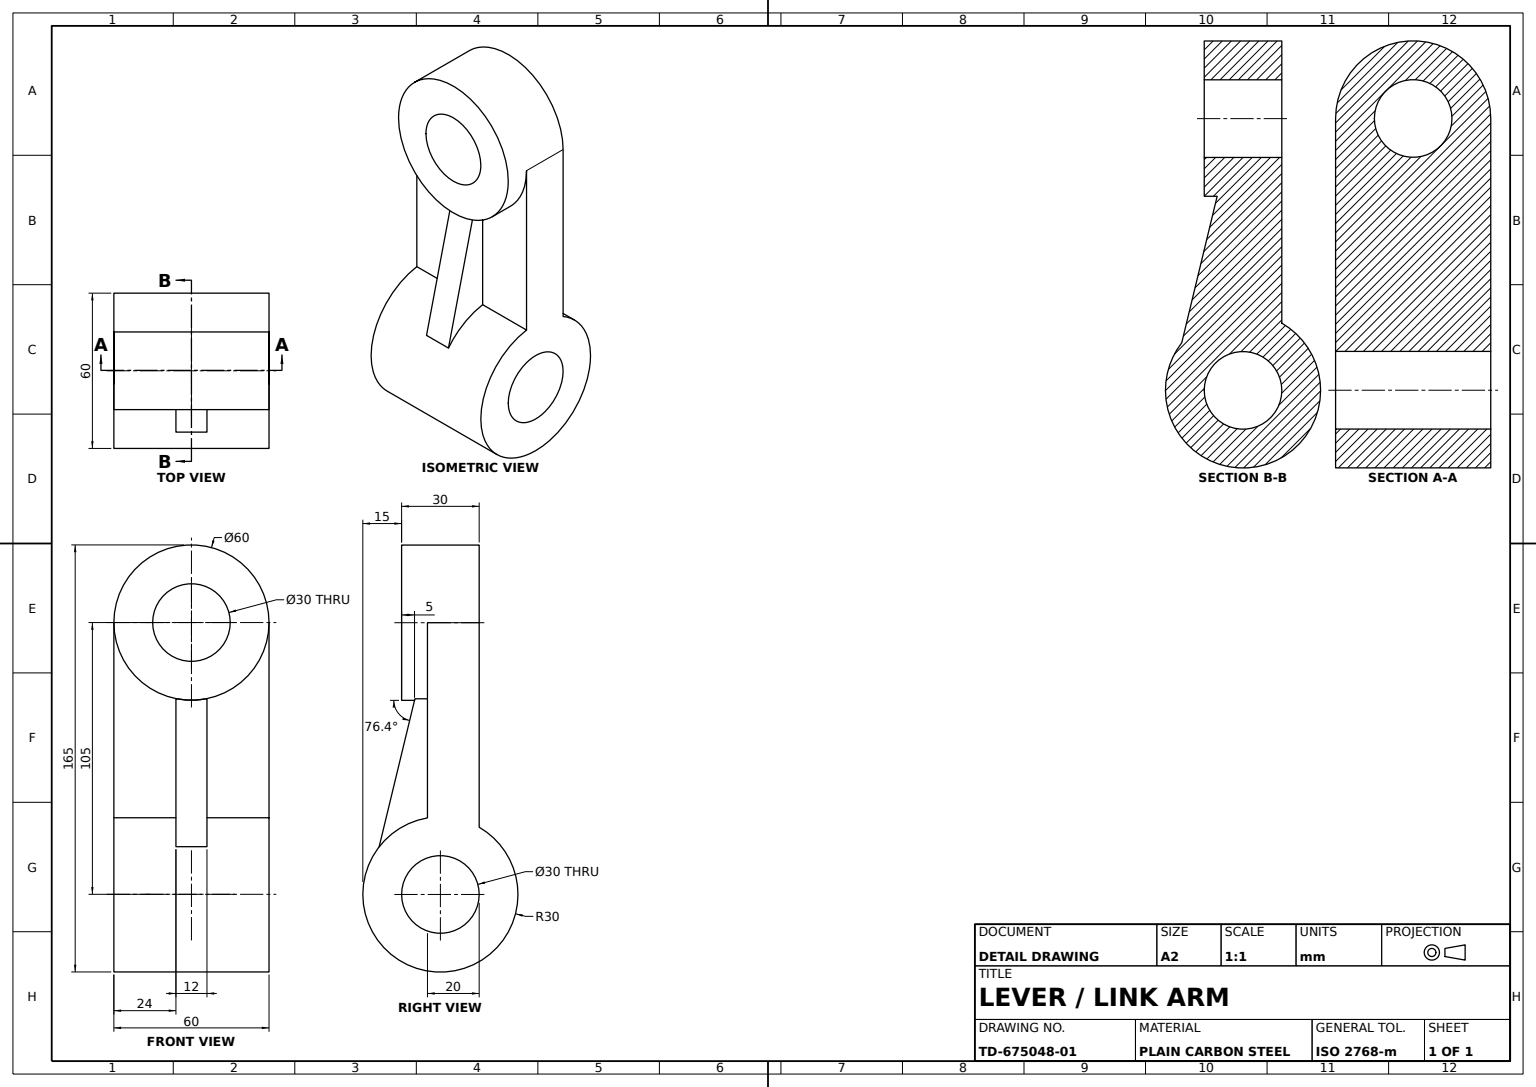
SolidWorks part; units mm, degrees
material "Plain Carbon Steel"
ref_plane "Front Plane" through (0, 0, 0) normal (0, 0, 1) x (1, 0, 0)
ref_plane "Top Plane" through (0, 0, 0) normal (0, 1, 0) x (1, 0, 0)
ref_plane "Right Plane" through (0, 0, 0) normal (1, 0, 0) x (0, 0, -1)
sketch "Upper Eye Sketch" plane through (0, 0, 0) normal (0, 0, 1) x (1, 0, 0)
  circle A0 centre (0, 0) radius 30
  dimension "D1" = 60
extrude "Upper Eye Boss" add sketch "Upper Eye Sketch" along normal blind 30
sketch "Upper Eye Bore Sketch" plane through (0, 0, 30) normal (0, 0, 1) x (1, 0, 0)
  circle A0 centre (0, 0) radius 15
  dimension "D1" = 30
extrude "Upper Eye Bore" cut sketch "Upper Eye Bore Sketch" against normal through all
sketch "Arm Profile Sketch" plane through (0, 0, 0) normal (1, 0, 0) x (0, 0, -1)
  line L2 (-20, 0) -> (-20, -80)
  line L3 (-20, -80) -> (0, -80)
  line L4 (0, -80) -> (0, 0)
  line L5 (0, 0) -> (-20, 0)
  dimension "D1" = 20
  dimension "D2" = 80
extrude "Arm" add sketch "Arm Profile Sketch" along normal mid plane 60
sketch "Arm Trim Sketch" plane through (0, 0, 0) normal (0, 0, 1) x (1, 0, 0)
  line L1 (15, 0) -> (-15, 0)
  line L2 (15, 0) -> (-15, 0)
  arc A1 (-15, 0) -> (15, 0) centre (0, 0) ccw
  arc A2 (-15, 0) -> (15, 0) centre (0, 0) ccw
  dimension "D1" = 0
extrude "Arm Trim Cut" cut sketch "Arm Trim Sketch" along normal blind 60
sketch "Lower Eye Sketch" plane through (0, 0, 0) normal (1, 0, 0) x (0, 0, -1)
  circle A1 centre (-15, -105) radius 30
  dimension "D1" = 60
  dimension "D2" = 15
  dimension "D3" = 105
extrude "Lower Eye Boss" add sketch "Lower Eye Sketch" along normal mid plane 60
sketch "Arm Rib Sketch" plane through (0, 0, 0) normal (1, 0, 0) x (0, 0, -1)
  line L0 (-25, -30) -> (-38.6944, -86.5996)
  line L1 (-30, -30) -> (-20, -30) construction
  arc A0 (-20, -75.4196) -> (0, -79.0192) centre (-15, -105) ccw construction
  dimension "D1" = 13.6944
rib "Arm Rib 12mm" sketch "Arm Rib Sketch" sketch "Arm Rib Sketch" thickness 12 extrusion direction parallel to sketch draft on no parameters "D1"=12
sketch "Lower Eye Bore Sketch" plane through (30, 0, 0) normal (1, 0, 0) x (0, 0, -1)
  circle A0 centre (-15, -105) radius 15
  dimension "D1" = 30
extrude "Lower Eye Bore" cut sketch "Lower Eye Bore Sketch" against normal through all
